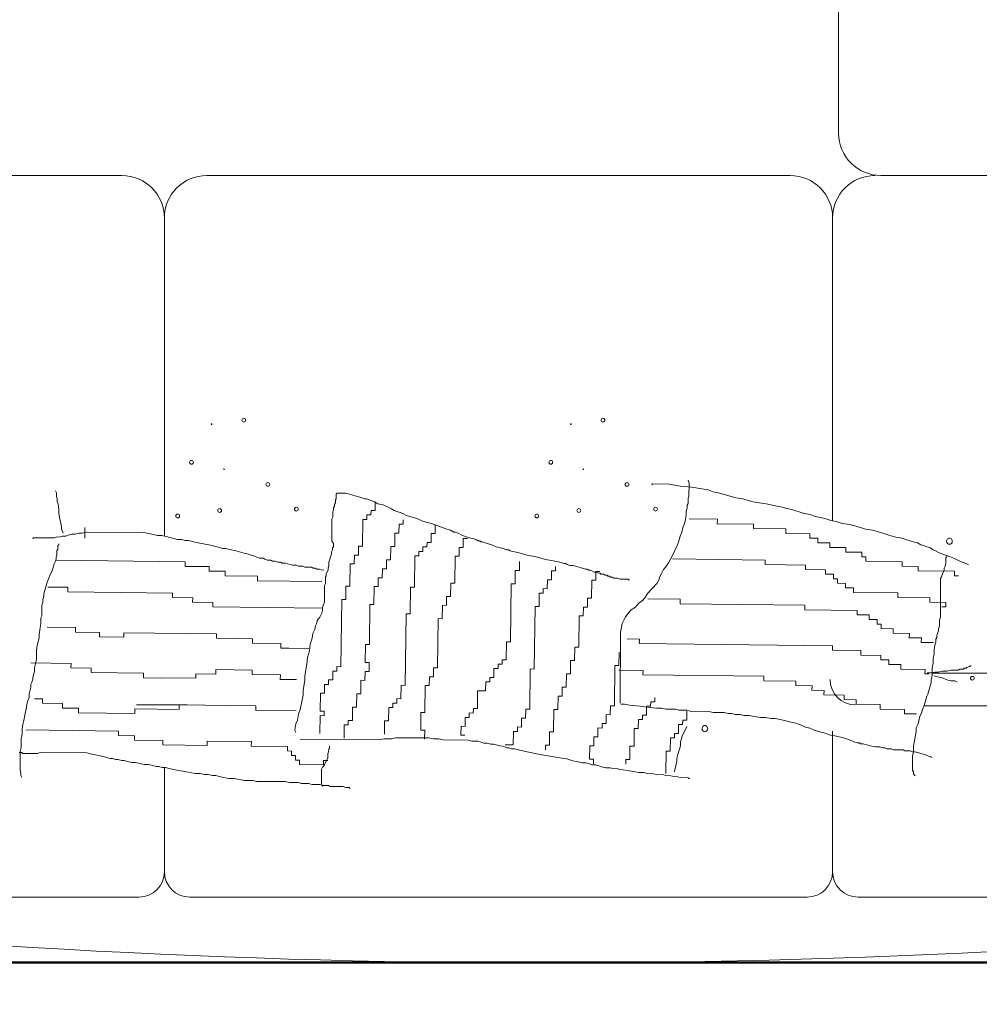
# Model space of a CAD drawing. Units: inches. Extents: x -466983 to 1020, y 324 to 318697.
# Tile 20 of 97: x 721 to 775, y 511 to 566. Entities that reach past the tile are written whole.
import ezdxf

# ---------------------------------------------------------------- set-up
doc = ezdxf.new("R2010")
doc.units = ezdxf.units.IN
doc.header["$MEASUREMENT"] = 0
for name, color, linetype, lineweight in [('A-ANNO-DIMS', 2, 'Continuous', 18), ('A-FURN', 8, 'Continuous', 18), ('A-WALL', 7, 'Continuous', 50)]:
    doc.layers.add(name, color=color, linetype=linetype, lineweight=lineweight)
doc.styles.get("Standard").update_dxf_attribs({"font": 'arial.ttf'})
doc.dimstyles.get("Standard").update_dxf_attribs({"dimtxt": 6, "dimasz": 4, "dimexe": 3, "dimexo": 3, "dimgap": 0.09, "dimtad": 0, "dimtih": 1, "dimtoh": 1, "dimdec": 1, "dimzin": 0, "dimdsep": 46, "dimlunit": 3, "dimtxsty": 'Standard', "dimcen": 0.09, "dimadec": 0, "dimazin": 0, "dimtfac": 1, "dimtdec": 1, "dimtofl": 0, "dimtmove": 0, "dimatfit": 3, "dimfxl": 1, "dimtolj": 1, "dimtzin": 0, "dimarcsym": 0})

# ---------------------------------------------------------------- blocks, each defined once
blk = doc.blocks.new('L Shaped Sofa')
at = {"ltscale": 2}
for p, q in [((2432.683, 769.955), (2432.683, 801.818)), ((2377.232, 767.567), (2392.324, 767.567)), ((2429.959, 767.567), (2397.1, 767.567)), ((2469.187, 767.567), (2435.071, 767.567)), ((2394.712, 747.255), (2394.712, 765.179)), ((2432.347, 748.121), (2432.347, 765.179)), ((2422.162, 750.193), (2423.138, 750.189)), ((2422.21, 750.139), (2422.162, 750.193)), ((2423.138, 750.189), (2423.772, 750.077)), ((2423.772, 750.077), (2424.406, 750.02)), ((2424.26, 750.238), (2424.213, 750.4)), ((2424.256, 749.479), (2424.26, 750.238)), ((2424.406, 750.02), (2424.747, 749.964)), ((2424.747, 749.964), (2425.332, 749.853)), ((2388.636, 749.7), (2388.588, 749.809)), ((2388.634, 749.483), (2388.636, 749.7)), ((2388.683, 749.374), (2388.634, 749.483)), ((2388.682, 749.212), (2388.683, 749.374)), ((2404.346, 749.301), (2404.395, 749.355)), ((2404.395, 749.355), (2404.397, 749.626)), ((2404.397, 749.626), (2404.446, 749.68)), ((2404.446, 749.68), (2404.934, 749.678)), ((2404.934, 749.678), (2405.713, 749.457)), ((2405.713, 749.457), (2406.005, 749.347)), ((2406.005, 749.347), (2406.103, 749.347)), ((2406.103, 749.347), (2406.541, 749.182)), ((2424.205, 749.099), (2424.206, 749.37)), ((2424.206, 749.37), (2424.256, 749.479)), ((2425.332, 749.853), (2425.624, 749.743)), ((2425.624, 749.743), (2425.916, 749.688)), ((2425.916, 749.688), (2426.89, 749.412)), ((2426.89, 749.412), (2427.28, 749.356)), ((2427.28, 749.356), (2427.865, 749.191)), ((2388.729, 749.049), (2388.682, 749.212)), ((2388.776, 748.778), (2388.729, 749.049)), ((2404.245, 748.759), (2404.246, 748.868)), ((2404.246, 748.868), (2404.295, 748.922)), ((2404.295, 749.03), (2404.345, 749.138)), ((2404.295, 748.922), (2404.295, 749.03)), ((2404.345, 749.138), (2404.346, 749.301)), ((2406.541, 749.182), (2406.735, 749.073)), ((2406.579, 748.695), (2406.585, 749.199)), ((2406.735, 749.073), (2407.028, 749.017)), ((2407.028, 749.017), (2407.514, 748.798)), ((2407.514, 748.798), (2407.66, 748.689)), ((2424.104, 748.666), (2424.154, 748.828)), ((2424.154, 748.828), (2424.155, 748.991)), ((2424.155, 748.991), (2424.205, 749.099)), ((2427.865, 749.191), (2428.206, 749.135)), ((2428.206, 749.135), (2428.596, 749.079)), ((2428.596, 749.079), (2429.132, 748.968)), ((2429.132, 748.968), (2429.425, 748.912)), ((2429.425, 748.912), (2429.766, 748.802)), ((2429.766, 748.802), (2430.058, 748.747)), ((2388.775, 748.507), (2388.776, 748.778)), ((2388.822, 748.235), (2388.775, 748.507)), ((2388.917, 747.801), (2388.822, 748.235)), ((2404.144, 748.218), (2404.193, 748.326)), ((2404.193, 748.326), (2404.195, 748.597)), ((2404.195, 748.597), (2404.245, 748.759)), ((2406.119, 748.197), (2406.122, 748.449)), ((2406.122, 748.449), (2406.349, 748.446)), ((2406.349, 748.446), (2406.352, 748.698)), ((2406.352, 748.698), (2406.579, 748.695)), ((2407.66, 748.689), (2407.806, 748.634)), ((2407.806, 748.634), (2408.001, 748.579)), ((2408.001, 748.579), (2408.147, 748.524)), ((2408.147, 748.524), (2408.342, 748.415)), ((2408.342, 748.415), (2408.926, 748.249)), ((2408.926, 748.249), (2409.072, 748.194)), ((2424.053, 748.178), (2424.103, 748.449)), ((2424.103, 748.449), (2424.104, 748.666)), ((2430.058, 748.747), (2430.74, 748.526)), ((2430.74, 748.526), (2431.081, 748.471)), ((2431.081, 748.471), (2431.373, 748.361)), ((2431.373, 748.361), (2431.666, 748.305)), ((2431.666, 748.305), (2431.909, 748.25)), ((2431.909, 748.25), (2432.25, 748.14)), ((2388.916, 747.638), (2388.917, 747.801)), ((2390.234, 747.741), (2390.23, 747.144)), ((2404.136, 746.971), (2404.144, 748.218)), ((2405.873, 746.688), (2405.892, 748.199)), ((2405.892, 748.199), (2406.119, 748.197)), ((2407.924, 747.419), (2407.93, 747.923)), ((2407.93, 747.923), (2408.157, 747.92)), ((2408.157, 747.92), (2408.16, 748.172)), ((2409.072, 748.194), (2409.17, 748.14)), ((2409.17, 748.14), (2409.316, 748.085)), ((2409.316, 748.085), (2409.51, 748.03)), ((2409.51, 748.03), (2409.754, 747.974)), ((2409.754, 747.974), (2410.63, 747.645)), ((2409.966, 747.394), (2409.972, 747.898)), ((2423.853, 747.474), (2423.904, 747.745)), ((2423.904, 747.745), (2424.003, 747.962)), ((2424.003, 747.962), (2424.053, 748.178)), ((2424.269, 748.227), (2425.857, 748.207)), ((2425.857, 748.207), (2425.853, 747.956)), ((2425.853, 747.956), (2427.895, 747.931)), ((2427.895, 747.931), (2427.892, 747.679)), ((2427.892, 747.679), (2429.707, 747.657)), ((2432.25, 748.14), (2432.543, 748.084)), ((2432.543, 748.084), (2432.884, 747.974)), ((2432.884, 747.974), (2433.322, 747.918)), ((2433.322, 747.918), (2433.858, 747.753)), ((2433.858, 747.753), (2434.199, 747.643)), ((2387.302, 747.104), (2387.351, 747.158)), ((2387.351, 747.158), (2388.523, 747.152)), ((2388.523, 747.152), (2388.669, 747.206)), ((2388.669, 747.206), (2388.816, 747.205)), ((2388.816, 747.205), (2388.962, 747.259)), ((2389.012, 747.421), (2388.916, 747.638)), ((2388.962, 747.259), (2389.158, 747.258)), ((2389.158, 747.258), (2389.304, 747.311)), ((2389.304, 747.311), (2389.5, 747.365)), ((2389.5, 747.365), (2389.695, 747.364)), ((2389.695, 747.364), (2389.89, 747.417)), ((2389.89, 747.417), (2390.086, 747.416)), ((2390.086, 747.416), (2390.33, 747.469)), ((2390.33, 747.469), (2393.55, 747.454)), ((2393.55, 747.454), (2393.843, 747.398)), ((2393.843, 747.398), (2394.33, 747.288)), ((2394.33, 747.288), (2394.574, 747.287)), ((2394.574, 747.287), (2394.818, 747.231)), ((2394.818, 747.231), (2395.013, 747.176)), ((2395.013, 747.176), (2395.256, 747.121)), ((2407.688, 746.666), (2407.697, 747.422)), ((2407.697, 747.422), (2407.924, 747.419)), ((2409.733, 746.893), (2409.739, 747.397)), ((2409.739, 747.397), (2409.966, 747.394)), ((2410.63, 747.645), (2410.825, 747.59)), ((2410.825, 747.59), (2411.02, 747.48)), ((2411.02, 747.48), (2411.117, 747.48)), ((2411.117, 747.48), (2411.263, 747.425)), ((2411.263, 747.425), (2411.458, 747.316)), ((2411.458, 747.316), (2411.701, 747.206)), ((2411.544, 746.619), (2411.55, 747.123)), ((2411.55, 747.123), (2411.777, 747.12)), ((2411.701, 747.206), (2411.896, 747.151)), ((2411.896, 747.151), (2412.14, 747.096)), ((2423.704, 747.041), (2423.754, 747.258)), ((2423.754, 747.258), (2423.853, 747.474)), ((2429.707, 747.657), (2429.704, 747.405)), ((2429.704, 747.405), (2431.065, 747.388)), ((2431.065, 747.388), (2431.061, 747.136)), ((2431.061, 747.136), (2431.515, 747.131)), ((2431.515, 747.131), (2431.512, 746.879)), ((2434.199, 747.643), (2434.589, 747.587)), ((2434.589, 747.587), (2435.174, 747.421)), ((2435.174, 747.421), (2435.515, 747.311)), ((2435.515, 747.311), (2435.904, 747.201)), ((2435.904, 747.201), (2436.246, 747.145)), ((2436.246, 747.145), (2436.586, 747.035)), ((2388.714, 746.501), (2388.715, 746.718)), ((2388.715, 746.718), (2388.764, 746.772)), ((2388.764, 746.772), (2388.765, 746.826)), ((2395.256, 747.121), (2395.451, 747.066)), ((2395.451, 747.066), (2395.695, 747.064)), ((2395.695, 747.064), (2395.89, 747.009)), ((2395.89, 747.009), (2396.085, 747.008)), ((2396.085, 747.008), (2396.28, 746.953)), ((2396.28, 746.953), (2396.524, 746.898)), ((2396.524, 746.898), (2397.401, 746.731)), ((2397.401, 746.731), (2397.596, 746.676)), ((2397.596, 746.676), (2397.839, 746.621)), ((2397.839, 746.621), (2397.985, 746.566)), ((2404.233, 746.862), (2404.136, 746.971)), ((2404.182, 746.482), (2404.183, 746.591)), ((2404.183, 746.591), (2404.232, 746.645)), ((2404.232, 746.645), (2404.233, 746.862)), ((2405.64, 746.187), (2405.647, 746.691)), ((2405.647, 746.691), (2405.873, 746.688)), ((2407.452, 745.913), (2407.461, 746.669)), ((2407.461, 746.669), (2407.688, 746.666)), ((2409.273, 746.394), (2409.276, 746.646)), ((2409.276, 746.646), (2409.503, 746.644)), ((2409.503, 746.644), (2409.506, 746.896)), ((2409.506, 746.896), (2409.733, 746.893)), ((2411.311, 746.118), (2411.317, 746.621)), ((2411.317, 746.621), (2411.544, 746.619)), ((2412.14, 747.096), (2412.286, 747.041)), ((2412.286, 747.041), (2412.383, 746.986)), ((2412.383, 746.986), (2412.481, 746.986)), ((2412.481, 746.986), (2412.529, 746.931)), ((2412.529, 746.931), (2412.627, 746.931)), ((2412.627, 746.931), (2412.773, 746.876)), ((2412.773, 746.876), (2413.162, 746.766)), ((2413.162, 746.766), (2413.406, 746.656)), ((2413.406, 746.656), (2413.649, 746.601)), ((2413.649, 746.601), (2413.844, 746.545)), ((2423.308, 746.122), (2423.605, 746.771)), ((2423.605, 746.771), (2423.704, 747.041)), ((2431.512, 746.879), (2432.193, 746.87)), ((2432.193, 746.87), (2432.19, 746.618)), ((2432.19, 746.618), (2433.097, 746.607)), ((2433.097, 746.607), (2433.094, 746.355)), ((2436.586, 747.035), (2436.879, 746.925)), ((2436.879, 746.925), (2437.122, 746.87)), ((2437.122, 746.87), (2437.317, 746.761)), ((2437.317, 746.761), (2437.512, 746.705)), ((2437.512, 746.705), (2437.658, 746.651)), ((2437.658, 746.651), (2437.852, 746.595)), ((2437.852, 746.595), (2437.998, 746.486)), ((2388.613, 745.959), (2388.614, 746.068)), ((2388.614, 746.068), (2388.663, 746.176)), ((2388.663, 746.176), (2388.665, 746.447)), ((2388.665, 746.447), (2388.714, 746.501)), ((2397.985, 746.566), (2398.181, 746.565)), ((2398.181, 746.565), (2398.57, 746.455)), ((2398.57, 746.455), (2398.814, 746.399)), ((2398.814, 746.399), (2399.204, 746.289)), ((2399.204, 746.289), (2399.447, 746.234)), ((2399.447, 746.234), (2399.593, 746.179)), ((2399.593, 746.179), (2399.788, 746.123)), ((2399.788, 746.123), (2400.08, 746.014)), ((2400.08, 746.014), (2400.276, 746.013)), ((2400.276, 746.013), (2400.373, 745.958)), ((2403.983, 745.779), (2404.132, 746.266)), ((2404.132, 746.266), (2404.133, 746.374)), ((2404.133, 746.374), (2404.182, 746.482)), ((2405.407, 745.686), (2405.414, 746.19)), ((2405.414, 746.19), (2405.64, 746.187)), ((2408.795, 744.385), (2408.816, 746.148)), ((2408.816, 746.148), (2409.043, 746.145)), ((2409.043, 746.145), (2409.046, 746.397)), ((2409.046, 746.397), (2409.273, 746.394)), ((2411.066, 744.609), (2411.084, 746.12)), ((2411.084, 746.12), (2411.311, 746.118)), ((2413.844, 746.545), (2413.99, 746.491)), ((2413.99, 746.491), (2414.088, 746.49)), ((2414.088, 746.49), (2414.185, 746.435)), ((2414.185, 746.435), (2414.331, 746.381)), ((2414.331, 746.381), (2414.624, 746.325)), ((2414.624, 746.325), (2415.208, 746.16)), ((2415.208, 746.16), (2415.598, 746.104)), ((2415.598, 746.104), (2416.183, 745.938)), ((2423.21, 745.959), (2423.308, 746.122)), ((2433.094, 746.355), (2434.001, 746.344)), ((2434.001, 746.344), (2433.998, 746.092)), ((2433.998, 746.092), (2434.225, 746.09)), ((2434.225, 746.09), (2434.222, 745.838)), ((2437.998, 746.486), (2438.144, 746.431)), ((2438.144, 746.431), (2438.339, 746.322)), ((2438.339, 746.322), (2438.582, 746.213)), ((2438.582, 746.213), (2438.923, 746.102)), ((2438.725, 745.724), (2438.727, 746.049)), ((2438.727, 746.049), (2438.777, 746.103)), ((2438.923, 746.102), (2439.215, 745.993)), ((2388.414, 745.364), (2388.514, 745.688)), ((2388.514, 745.688), (2388.563, 745.797)), ((2388.563, 745.797), (2388.613, 745.959)), ((2388.622, 745.891), (2395.88, 745.802)), ((2395.88, 745.802), (2395.877, 745.55)), ((2395.877, 745.55), (2397.238, 745.534)), ((2397.238, 745.534), (2397.235, 745.282)), ((2400.373, 745.958), (2400.519, 745.903)), ((2400.519, 745.903), (2400.714, 745.902)), ((2400.714, 745.902), (2400.811, 745.848)), ((2400.811, 745.848), (2400.958, 745.847)), ((2400.958, 745.847), (2401.104, 745.792)), ((2401.104, 745.792), (2401.25, 745.791)), ((2401.25, 745.791), (2401.347, 745.737)), ((2401.347, 745.737), (2401.543, 745.736)), ((2401.543, 745.736), (2401.932, 745.625)), ((2401.932, 745.625), (2402.127, 745.625)), ((2402.127, 745.625), (2402.273, 745.57)), ((2402.273, 745.57), (2402.517, 745.569)), ((2402.517, 745.569), (2402.615, 745.514)), ((2402.615, 745.514), (2403.005, 745.512)), ((2403.005, 745.512), (2403.102, 745.457)), ((2403.102, 745.457), (2403.2, 745.457)), ((2403.2, 745.457), (2403.297, 745.402)), ((2403.932, 745.453), (2403.982, 745.616)), ((2403.982, 745.616), (2403.983, 745.779)), ((2405.165, 744.429), (2405.181, 745.689)), ((2405.181, 745.689), (2405.407, 745.686)), ((2407.219, 745.412), (2407.225, 745.916)), ((2407.225, 745.916), (2407.452, 745.913)), ((2414.705, 745.32), (2414.711, 745.824)), ((2416.183, 745.938), (2416.524, 745.882)), ((2416.524, 745.882), (2416.816, 745.827)), ((2416.746, 745.295), (2416.749, 745.547)), ((2416.816, 745.827), (2417.06, 745.771)), ((2417.06, 745.771), (2417.206, 745.716)), ((2417.206, 745.716), (2417.304, 745.716)), ((2417.304, 745.716), (2417.401, 745.661)), ((2417.401, 745.661), (2417.547, 745.606)), ((2417.547, 745.606), (2417.742, 745.605)), ((2417.742, 745.605), (2418.132, 745.495)), ((2418.132, 745.495), (2418.424, 745.385)), ((2422.816, 745.365), (2422.963, 745.527)), ((2422.963, 745.527), (2423.111, 745.743)), ((2423.111, 745.743), (2423.21, 745.959)), ((2423.334, 745.971), (2428.551, 745.907)), ((2428.551, 745.907), (2428.548, 745.655)), ((2428.548, 745.655), (2430.816, 745.627)), ((2430.816, 745.627), (2430.813, 745.375)), ((2434.222, 745.838), (2436.263, 745.813)), ((2436.263, 745.813), (2436.26, 745.561)), ((2436.26, 745.561), (2437.168, 745.55)), ((2437.168, 745.55), (2437.165, 745.298)), ((2438.626, 745.453), (2438.676, 745.561)), ((2438.676, 745.561), (2438.725, 745.724)), ((2439.215, 745.993), (2439.556, 745.828)), ((2439.556, 745.828), (2439.994, 745.664)), ((2388.216, 744.877), (2388.266, 745.039)), ((2388.266, 745.039), (2388.414, 745.364)), ((2397.235, 745.282), (2398.143, 745.271)), ((2398.143, 745.271), (2398.139, 745.019)), ((2398.139, 745.019), (2399.954, 744.997)), ((2399.954, 744.997), (2399.951, 744.745)), ((2403.297, 745.402), (2403.444, 745.402)), ((2403.444, 745.402), (2403.541, 745.347)), ((2403.541, 745.347), (2403.687, 745.346)), ((2403.78, 744.587), (2403.782, 744.966)), ((2403.782, 744.966), (2403.832, 745.02)), ((2403.832, 745.129), (2403.931, 745.345)), ((2403.832, 745.02), (2403.832, 745.129)), ((2403.931, 745.345), (2403.932, 745.453)), ((2406.753, 744.41), (2406.759, 744.914)), ((2406.759, 744.914), (2406.986, 744.911)), ((2406.986, 744.911), (2406.992, 745.415)), ((2406.992, 745.415), (2407.219, 745.412)), ((2414.469, 744.567), (2414.478, 745.323)), ((2414.478, 745.323), (2414.705, 745.32)), ((2416.513, 744.794), (2416.519, 745.298)), ((2416.519, 745.298), (2416.746, 745.295)), ((2418.424, 745.385), (2418.522, 745.385)), ((2418.522, 745.385), (2418.619, 745.33)), ((2418.619, 745.33), (2418.716, 745.33)), ((2418.716, 745.33), (2418.911, 745.22)), ((2418.911, 745.22), (2419.057, 745.22)), ((2419.008, 744.764), (2419.015, 745.268)), ((2419.015, 745.268), (2419.241, 745.265)), ((2419.057, 745.22), (2419.155, 745.165)), ((2419.155, 745.165), (2419.252, 745.165)), ((2419.252, 745.165), (2419.301, 745.11)), ((2419.301, 745.11), (2419.447, 745.11)), ((2419.447, 745.11), (2419.544, 745.055)), ((2419.544, 745.055), (2419.642, 745.054)), ((2419.642, 745.054), (2419.69, 745)), ((2419.69, 745), (2419.788, 744.999)), ((2419.788, 744.999), (2419.836, 744.945)), ((2419.836, 744.945), (2419.934, 744.945)), ((2419.934, 744.945), (2420.031, 744.89)), ((2422.568, 744.77), (2422.618, 744.986)), ((2422.618, 744.986), (2422.717, 745.148)), ((2422.717, 745.148), (2422.816, 745.365)), ((2430.813, 745.375), (2431.947, 745.362)), ((2431.947, 745.362), (2431.944, 745.11)), ((2431.944, 745.11), (2432.398, 745.104)), ((2432.398, 745.104), (2432.395, 744.852)), ((2437.165, 745.298), (2439.206, 745.273)), ((2438.427, 744.858), (2438.477, 744.966)), ((2438.477, 744.966), (2438.527, 745.128)), ((2438.527, 745.128), (2438.626, 745.345)), ((2438.626, 745.345), (2438.626, 745.453)), ((2439.206, 745.273), (2439.203, 745.021)), ((2439.43, 745.018), (2439.203, 745.021)), ((2439.203, 745.021), (2439.43, 745.018)), ((2387.918, 744.011), (2388.117, 744.66)), ((2388.117, 744.66), (2388.216, 744.877)), ((2388.149, 744.385), (2389.284, 744.371)), ((2389.284, 744.371), (2389.281, 744.119)), ((2399.951, 744.745), (2403.58, 744.7)), ((2403.725, 743.557), (2403.731, 744.478)), ((2403.731, 744.478), (2403.78, 744.587)), ((2404.929, 743.676), (2404.938, 744.432)), ((2404.938, 744.432), (2405.165, 744.429)), ((2406.514, 743.405), (2406.526, 744.412)), ((2406.526, 744.412), (2406.753, 744.41)), ((2408.549, 742.876), (2408.568, 744.388)), ((2408.568, 744.388), (2408.795, 744.385)), ((2410.83, 743.856), (2410.839, 744.612)), ((2410.839, 744.612), (2411.066, 744.609)), ((2414.202, 741.295), (2414.242, 744.57)), ((2414.242, 744.57), (2414.469, 744.567)), ((2416.28, 744.293), (2416.286, 744.797)), ((2416.286, 744.797), (2416.513, 744.794)), ((2418.769, 743.759), (2418.782, 744.767)), ((2418.782, 744.767), (2419.008, 744.764)), ((2420.031, 744.89), (2420.226, 744.889)), ((2420.226, 744.889), (2420.372, 744.834)), ((2420.372, 744.834), (2420.812, 744.832)), ((2420.812, 744.832), (2420.909, 744.777)), ((2421.929, 744.014), (2422.469, 744.607)), ((2422.469, 744.607), (2422.568, 744.77)), ((2432.395, 744.852), (2432.622, 744.849)), ((2432.622, 744.849), (2432.619, 744.598)), ((2432.619, 744.598), (2433.072, 744.592)), ((2433.072, 744.592), (2433.069, 744.34)), ((2438.414, 742.689), (2438.427, 744.858)), ((2387.867, 743.685), (2387.917, 743.848)), ((2387.917, 743.848), (2387.918, 744.011)), ((2389.281, 744.119), (2395.178, 744.047)), ((2395.178, 744.047), (2395.175, 743.795)), ((2395.175, 743.795), (2396.309, 743.781)), ((2410.597, 743.355), (2410.603, 743.859)), ((2410.603, 743.859), (2410.83, 743.856)), ((2415.814, 743.291), (2415.823, 744.047)), ((2415.823, 744.047), (2416.05, 744.044)), ((2416.05, 744.044), (2416.053, 744.296)), ((2416.053, 744.296), (2416.28, 744.293)), ((2421.634, 743.635), (2421.781, 743.797)), ((2421.781, 743.797), (2421.929, 744.014)), ((2433.069, 744.34), (2433.523, 744.335)), ((2433.523, 744.335), (2433.52, 744.083)), ((2433.52, 744.083), (2436.015, 744.052)), ((2436.015, 744.052), (2436.012, 743.8)), ((2436.012, 743.8), (2437.827, 743.778)), ((2387.813, 742.764), (2387.816, 743.36)), ((2387.816, 743.36), (2387.866, 743.523)), ((2387.866, 743.523), (2387.867, 743.685)), ((2396.309, 743.781), (2396.306, 743.53)), ((2396.306, 743.53), (2397.44, 743.516)), ((2397.44, 743.516), (2397.437, 743.264)), ((2397.437, 743.264), (2403.562, 743.189)), ((2403.625, 743.232), (2403.725, 743.557)), ((2404.656, 739.9), (2404.702, 743.679)), ((2404.702, 743.679), (2404.929, 743.676)), ((2406.259, 741.14), (2406.287, 743.408)), ((2406.287, 743.408), (2406.514, 743.405)), ((2410.361, 742.602), (2410.37, 743.358)), ((2410.37, 743.358), (2410.597, 743.355)), ((2415.544, 739.767), (2415.587, 743.294)), ((2415.587, 743.294), (2415.814, 743.291)), ((2418.303, 742.757), (2418.309, 743.261)), ((2418.309, 743.261), (2418.536, 743.258)), ((2418.536, 743.258), (2418.542, 743.762)), ((2418.542, 743.762), (2418.769, 743.759)), ((2420.996, 743.096), (2421.241, 743.258)), ((2421.241, 743.258), (2421.438, 743.474)), ((2421.438, 743.474), (2421.634, 743.635)), ((2421.945, 743.72), (2423.76, 743.698)), ((2423.76, 743.698), (2423.757, 743.446)), ((2423.757, 743.446), (2430.788, 743.36)), ((2430.788, 743.36), (2430.785, 743.108)), ((2437.827, 743.778), (2437.823, 743.526)), ((2437.823, 743.526), (2438.731, 743.515)), ((2438.728, 743.263), (2438.501, 743.266)), ((2438.731, 743.515), (2438.728, 743.263)), ((2387.763, 742.656), (2387.813, 742.764)), ((2403.378, 742.583), (2403.476, 742.69)), ((2403.476, 742.69), (2403.575, 742.907)), ((2403.575, 742.907), (2403.624, 743.069)), ((2403.624, 743.069), (2403.625, 743.232)), ((2408.273, 738.848), (2408.322, 742.879)), ((2408.322, 742.879), (2408.549, 742.876)), ((2418.055, 740.996), (2418.076, 742.76)), ((2418.076, 742.76), (2418.303, 742.757)), ((2420.603, 742.556), (2420.701, 742.718)), ((2420.701, 742.718), (2420.849, 742.934)), ((2420.849, 742.934), (2420.996, 743.096)), ((2430.785, 743.108), (2433.734, 743.072)), ((2433.734, 743.072), (2433.731, 742.82)), ((2433.731, 742.82), (2434.412, 742.812)), ((2434.412, 742.812), (2434.409, 742.56)), ((2438.364, 742.527), (2438.414, 742.689)), ((2387.711, 742.114), (2387.761, 742.331)), ((2387.761, 742.331), (2387.763, 742.656)), ((2403.179, 741.987), (2403.229, 742.204)), ((2403.229, 742.204), (2403.278, 742.312)), ((2403.278, 742.312), (2403.328, 742.474)), ((2403.328, 742.474), (2403.378, 742.583)), ((2410.1, 739.834), (2410.134, 742.605)), ((2410.134, 742.605), (2410.361, 742.602)), ((2420.453, 742.123), (2420.504, 742.339)), ((2420.504, 742.339), (2420.603, 742.556)), ((2434.409, 742.56), (2434.862, 742.555)), ((2434.862, 742.555), (2434.859, 742.303)), ((2434.859, 742.303), (2435.086, 742.3)), ((2435.086, 742.3), (2435.083, 742.048)), ((2438.312, 742.039), (2438.362, 742.201)), ((2438.362, 742.201), (2438.364, 742.527)), ((2387.659, 741.518), (2387.66, 741.735)), ((2387.66, 741.735), (2387.71, 741.951)), ((2387.71, 741.951), (2387.711, 742.114)), ((2388.122, 742.118), (2389.71, 742.098)), ((2389.71, 742.098), (2389.706, 741.847)), ((2389.706, 741.847), (2391.067, 741.83)), ((2391.067, 741.83), (2391.064, 741.578)), ((2391.064, 741.578), (2392.425, 741.561)), ((2392.425, 741.561), (2392.429, 741.813)), ((2392.429, 741.813), (2397.646, 741.75)), ((2397.646, 741.75), (2397.643, 741.498)), ((2403.029, 741.5), (2403.08, 741.771)), ((2403.08, 741.771), (2403.179, 741.987)), ((2420.378, 737.84), (2420.403, 741.852)), ((2420.403, 741.852), (2420.453, 742.123)), ((2435.083, 742.048), (2435.764, 742.04)), ((2435.764, 742.04), (2435.76, 741.788)), ((2435.76, 741.788), (2436.668, 741.777)), ((2436.668, 741.777), (2436.665, 741.525)), ((2438.212, 741.552), (2438.213, 741.66)), ((2438.213, 741.66), (2438.262, 741.768)), ((2438.262, 741.768), (2438.312, 741.931)), ((2438.312, 741.931), (2438.312, 742.039)), ((2387.508, 740.814), (2387.558, 741.084)), ((2387.558, 741.084), (2387.659, 741.518)), ((2397.643, 741.498), (2399.684, 741.473)), ((2399.684, 741.473), (2399.681, 741.221)), ((2399.681, 741.221), (2401.269, 741.201)), ((2401.269, 741.201), (2401.266, 740.949)), ((2402.879, 740.796), (2402.93, 741.175)), ((2402.93, 741.175), (2403.029, 741.5)), ((2406.02, 740.135), (2406.033, 741.143)), ((2406.033, 741.143), (2406.259, 741.14)), ((2413.963, 740.29), (2413.975, 741.298)), ((2413.975, 741.298), (2414.202, 741.295)), ((2420.783, 741.467), (2421.464, 741.459)), ((2421.464, 741.459), (2421.46, 741.207)), ((2421.46, 741.207), (2432.349, 741.074)), ((2432.349, 741.074), (2432.346, 740.822)), ((2436.665, 741.525), (2437.345, 741.516)), ((2437.345, 741.516), (2437.342, 741.265)), ((2437.342, 741.265), (2438.023, 741.256)), ((2438.061, 740.847), (2438.112, 741.118)), ((2438.112, 741.118), (2438.161, 741.281)), ((2438.161, 741.281), (2438.162, 741.443)), ((2438.162, 741.443), (2438.212, 741.552)), ((2387.505, 740.326), (2387.508, 740.814)), ((2401.266, 740.949), (2401.72, 740.944)), ((2401.493, 740.947), (2402.854, 740.93)), ((2401.72, 740.944), (2401.493, 740.947)), ((2402.779, 740.417), (2402.879, 740.796)), ((2417.819, 740.243), (2417.828, 740.999)), ((2417.828, 740.999), (2418.055, 740.996)), ((2420.311, 739.961), (2420.32, 740.717)), ((2432.346, 740.822), (2433.933, 740.802)), ((2433.933, 740.802), (2433.93, 740.55)), ((2433.93, 740.55), (2435.065, 740.536)), ((2435.065, 740.536), (2435.061, 740.285)), ((2438.009, 740.36), (2438.06, 740.631)), ((2438.06, 740.631), (2438.061, 740.847)), ((2387.19, 740.114), (2389.458, 740.086)), ((2387.404, 739.838), (2387.454, 740.055)), ((2387.454, 740.055), (2387.505, 740.326)), ((2389.458, 740.086), (2389.455, 739.834)), ((2402.626, 739.387), (2402.728, 740.037)), ((2402.728, 740.037), (2402.779, 740.417)), ((2406.247, 740.133), (2406.02, 740.135)), ((2406.241, 739.629), (2406.247, 740.133)), ((2413.503, 739.792), (2413.506, 740.044)), ((2413.506, 740.044), (2413.733, 740.041)), ((2413.733, 740.041), (2413.736, 740.293)), ((2413.736, 740.293), (2413.963, 740.29)), ((2417.583, 739.49), (2417.592, 740.246)), ((2417.592, 740.246), (2417.819, 740.243)), ((2420.056, 737.696), (2420.084, 739.964)), ((2420.084, 739.964), (2420.311, 739.961)), ((2435.061, 740.285), (2435.515, 740.279)), ((2435.515, 740.279), (2435.512, 740.027)), ((2435.512, 740.027), (2436.193, 740.019)), ((2436.193, 740.019), (2436.189, 739.767)), ((2437.957, 739.818), (2438.008, 740.089)), ((2438.008, 740.089), (2438.009, 740.36)), ((2439.909, 739.863), (2440.056, 739.916)), ((2440.056, 739.916), (2440.154, 739.97)), ((2387.303, 739.296), (2387.403, 739.621)), ((2387.403, 739.621), (2387.404, 739.838)), ((2389.455, 739.834), (2390.589, 739.82)), ((2390.589, 739.82), (2390.586, 739.568)), ((2390.586, 739.568), (2393.535, 739.532)), ((2393.535, 739.532), (2393.532, 739.28)), ((2396.481, 739.244), (2396.484, 739.496)), ((2396.484, 739.496), (2397.618, 739.482)), ((2397.618, 739.482), (2397.621, 739.734)), ((2397.621, 739.734), (2399.663, 739.709)), ((2399.663, 739.709), (2399.66, 739.457)), ((2399.66, 739.457), (2401.247, 739.438)), ((2401.247, 739.438), (2401.244, 739.186)), ((2402.624, 739.116), (2402.626, 739.387)), ((2404.193, 739.15), (2404.199, 739.654)), ((2404.199, 739.654), (2404.426, 739.651)), ((2404.426, 739.651), (2404.429, 739.903)), ((2404.429, 739.903), (2404.656, 739.9)), ((2406.008, 739.128), (2406.014, 739.632)), ((2406.014, 739.632), (2406.241, 739.629)), ((2409.867, 739.333), (2409.873, 739.836)), ((2409.873, 739.836), (2410.1, 739.834)), ((2413.27, 739.291), (2413.276, 739.795)), ((2413.276, 739.795), (2413.503, 739.792)), ((2415.29, 737.503), (2415.317, 739.77)), ((2415.317, 739.77), (2415.544, 739.767)), ((2417.347, 738.737), (2417.356, 739.493)), ((2417.356, 739.493), (2417.583, 739.49)), ((2420.308, 739.709), (2421.669, 739.692)), ((2421.669, 739.692), (2421.666, 739.44)), ((2421.666, 739.44), (2428.471, 739.357)), ((2428.471, 739.357), (2428.468, 739.105)), ((2436.189, 739.767), (2437.55, 739.75)), ((2437.55, 739.75), (2437.547, 739.498)), ((2437.547, 739.498), (2437.774, 739.496)), ((2437.663, 739.548), (2437.907, 739.547)), ((2437.905, 739.167), (2437.955, 739.384)), ((2437.907, 739.547), (2438.102, 739.6)), ((2437.955, 739.384), (2437.957, 739.818)), ((2458.96, 739.532), (2437.956, 739.532)), ((2438.052, 739.384), (2438.247, 739.328)), ((2438.102, 739.6), (2438.298, 739.599)), ((2438.298, 739.599), (2438.542, 739.652)), ((2438.542, 739.652), (2438.786, 739.651)), ((2438.786, 739.651), (2439.03, 739.704)), ((2439.03, 739.704), (2439.42, 739.702)), ((2439.42, 739.702), (2439.518, 739.756)), ((2439.518, 739.756), (2439.714, 739.755)), ((2439.714, 739.755), (2439.763, 739.809)), ((2439.763, 739.809), (2439.86, 739.809)), ((2439.86, 739.809), (2439.909, 739.863)), ((2387.202, 738.755), (2387.203, 738.917)), ((2387.203, 738.917), (2387.253, 739.026)), ((2387.253, 739.026), (2387.303, 739.188)), ((2387.303, 739.188), (2387.303, 739.296)), ((2393.532, 739.28), (2396.481, 739.244)), ((2394.569, 739.178), (2394.569, 739.178)), ((2401.244, 739.186), (2402.152, 739.175)), ((2402.523, 738.574), (2402.624, 739.116)), ((2403.73, 738.4), (2403.736, 738.904)), ((2403.736, 738.904), (2403.963, 738.901)), ((2403.963, 738.901), (2403.966, 739.153)), ((2403.966, 739.153), (2404.193, 739.15)), ((2405.772, 738.375), (2405.781, 739.131)), ((2405.781, 739.131), (2406.008, 739.128)), ((2408.037, 738.095), (2408.046, 738.851)), ((2408.046, 738.851), (2408.273, 738.848)), ((2409.389, 737.323), (2409.407, 738.834)), ((2409.407, 738.834), (2409.634, 738.832)), ((2409.634, 738.832), (2409.64, 739.335)), ((2409.64, 739.335), (2409.867, 739.333)), ((2412.807, 738.541), (2412.813, 739.045)), ((2412.813, 739.045), (2413.04, 739.042)), ((2413.04, 739.042), (2413.043, 739.294)), ((2413.043, 739.294), (2413.27, 739.291)), ((2428.468, 739.105), (2430.282, 739.083)), ((2430.282, 739.083), (2430.279, 738.831)), ((2430.279, 738.831), (2431.187, 738.82)), ((2431.187, 738.82), (2431.184, 738.568)), ((2437.704, 738.355), (2437.904, 739.005)), ((2437.904, 739.005), (2437.905, 739.167)), ((2438.247, 739.328), (2438.54, 739.273)), ((2438.54, 739.273), (2438.783, 739.163)), ((2438.783, 739.163), (2439.026, 739.108)), ((2439.026, 739.108), (2439.222, 739.107)), ((2439.222, 739.107), (2439.368, 739.052)), ((2387.101, 738.159), (2387.103, 738.376)), ((2387.103, 738.376), (2387.153, 738.592)), ((2387.153, 738.592), (2387.202, 738.755)), ((2402.37, 737.491), (2402.522, 738.303)), ((2402.522, 738.303), (2402.523, 738.574)), ((2403.491, 737.395), (2403.503, 738.403)), ((2403.503, 738.403), (2403.73, 738.4)), ((2405.536, 737.622), (2405.545, 738.378)), ((2405.545, 738.378), (2405.772, 738.375)), ((2412.341, 737.539), (2412.353, 738.546)), ((2412.353, 738.546), (2412.807, 738.541)), ((2417.114, 738.236), (2417.12, 738.74)), ((2417.12, 738.74), (2417.347, 738.737)), ((2431.184, 738.568), (2431.864, 738.56)), ((2431.864, 738.56), (2431.861, 738.308)), ((2431.861, 738.308), (2432.995, 738.294)), ((2432.995, 738.294), (2432.992, 738.042)), ((2437.605, 738.03), (2437.655, 738.247)), ((2437.655, 738.247), (2437.704, 738.355)), ((2386.8, 736.859), (2387.002, 737.942)), ((2387.002, 737.942), (2387.101, 738.159)), ((2387.392, 738.096), (2387.846, 738.09)), ((2387.846, 738.09), (2387.843, 737.838)), ((2387.843, 737.838), (2388.977, 737.824)), ((2388.977, 737.824), (2388.974, 737.572)), ((2396.001, 737.746), (2393.136, 737.746)), ((2395.552, 737.492), (2395.555, 737.744)), ((2395.555, 737.744), (2399.865, 737.691)), ((2407.577, 737.597), (2407.58, 737.849)), ((2407.58, 737.849), (2407.807, 737.846)), ((2407.807, 737.846), (2407.81, 738.098)), ((2407.81, 738.098), (2408.037, 738.095)), ((2416.878, 737.483), (2416.887, 738.239)), ((2416.887, 738.239), (2417.114, 738.236)), ((2419.823, 737.195), (2419.83, 737.699)), ((2419.83, 737.699), (2420.056, 737.696)), ((2420.427, 737.786), (2420.622, 737.785)), ((2420.622, 737.785), (2420.915, 737.729)), ((2420.915, 737.729), (2421.5, 737.672)), ((2422.098, 737.672), (2422.101, 737.923)), ((2422.101, 737.923), (2422.328, 737.921)), ((2422.328, 737.921), (2422.331, 738.173)), ((2432.992, 738.042), (2433.673, 738.034)), ((2433.673, 738.034), (2433.67, 737.782)), ((2433.67, 737.782), (2435.031, 737.765)), ((2435.031, 737.765), (2435.028, 737.514)), ((2437.406, 737.489), (2437.505, 737.705)), ((2460.8, 737.692), (2437.499, 737.692)), ((2437.505, 737.705), (2437.605, 738.03)), ((2388.974, 737.572), (2389.881, 737.561)), ((2389.881, 737.561), (2389.878, 737.309)), ((2389.878, 737.309), (2393.054, 737.271)), ((2393.054, 737.271), (2393.057, 737.522)), ((2393.057, 737.522), (2395.552, 737.492)), ((2399.865, 737.691), (2399.862, 737.439)), ((2399.862, 737.439), (2402.13, 737.412)), ((2402.22, 736.895), (2402.271, 737.22)), ((2402.271, 737.22), (2402.37, 737.491)), ((2403.476, 736.135), (2403.488, 737.143)), ((2403.488, 737.143), (2403.715, 737.14)), ((2403.718, 737.392), (2403.491, 737.395)), ((2403.715, 737.14), (2403.718, 737.392)), ((2405.3, 736.869), (2405.309, 737.625)), ((2405.309, 737.625), (2405.536, 737.622)), ((2407.341, 736.844), (2407.35, 737.6)), ((2407.35, 737.6), (2407.577, 737.597)), ((2409.15, 736.318), (2409.162, 737.326)), ((2409.162, 737.326), (2409.389, 737.323)), ((2411.881, 737.041), (2411.884, 737.292)), ((2411.884, 737.292), (2412.111, 737.29)), ((2412.111, 737.29), (2412.114, 737.542)), ((2412.114, 737.542), (2412.341, 737.539)), ((2415.057, 737.002), (2415.063, 737.506)), ((2415.063, 737.506), (2415.29, 737.503)), ((2416.635, 736.227), (2416.651, 737.486)), ((2416.651, 737.486), (2416.878, 737.483)), ((2419.59, 736.694), (2419.597, 737.198)), ((2419.597, 737.198), (2419.823, 737.195)), ((2421.5, 737.672), (2421.89, 737.616)), ((2421.635, 736.921), (2421.638, 737.173)), ((2421.638, 737.173), (2421.865, 737.17)), ((2421.865, 737.17), (2421.871, 737.674)), ((2421.871, 737.674), (2422.098, 737.672)), ((2421.89, 737.616), (2422.426, 737.559)), ((2422.426, 737.559), (2422.719, 737.558)), ((2422.719, 737.558), (2422.963, 737.503)), ((2422.963, 737.503), (2423.499, 737.5)), ((2423.499, 737.5), (2423.694, 737.445)), ((2423.694, 737.445), (2424.133, 737.443)), ((2424.13, 736.891), (2424.136, 737.395)), ((2424.133, 737.443), (2424.328, 737.388)), ((2424.328, 737.388), (2425.353, 737.383)), ((2425.353, 737.383), (2425.645, 737.327)), ((2425.645, 737.327), (2426.231, 737.325)), ((2426.231, 737.325), (2426.475, 737.269)), ((2426.475, 737.269), (2426.67, 737.268)), ((2426.67, 737.268), (2426.865, 737.213)), ((2426.865, 737.213), (2427.157, 737.212)), ((2427.157, 737.212), (2427.352, 737.157)), ((2427.352, 737.157), (2427.645, 737.155)), ((2427.645, 737.155), (2427.937, 737.1)), ((2435.028, 737.514), (2436.389, 737.497)), ((2436.389, 737.497), (2436.386, 737.245)), ((2436.386, 737.245), (2437.066, 737.237)), ((2437.258, 737.11), (2437.356, 737.272)), ((2437.356, 737.272), (2437.406, 737.489)), ((2386.7, 736.372), (2386.75, 736.642)), ((2386.75, 736.642), (2386.8, 736.859)), ((2402.071, 736.462), (2402.121, 736.679)), ((2402.121, 736.679), (2402.22, 736.895)), ((2404.834, 735.867), (2404.843, 736.623)), ((2404.843, 736.623), (2405.07, 736.62)), ((2405.07, 736.62), (2405.073, 736.872)), ((2405.073, 736.872), (2405.3, 736.869)), ((2407.105, 736.091), (2407.114, 736.847)), ((2407.114, 736.847), (2407.341, 736.844)), ((2411.648, 736.539), (2411.654, 737.043)), ((2411.654, 737.043), (2411.881, 737.041)), ((2414.824, 736.501), (2414.83, 737.004)), ((2414.83, 737.004), (2415.057, 737.002)), ((2419.36, 736.445), (2419.364, 736.697)), ((2419.364, 736.697), (2419.59, 736.694)), ((2421.402, 736.42), (2421.408, 736.924)), ((2421.408, 736.924), (2421.635, 736.921)), ((2423.667, 736.141), (2423.673, 736.644)), ((2423.673, 736.644), (2423.9, 736.642)), ((2423.9, 736.642), (2423.903, 736.894)), ((2423.903, 736.894), (2424.13, 736.891)), ((2427.937, 737.1), (2428.279, 737.044)), ((2428.279, 737.044), (2428.571, 737.043)), ((2428.571, 737.043), (2428.864, 736.987)), ((2428.864, 736.987), (2429.108, 736.986)), ((2429.108, 736.986), (2429.4, 736.93)), ((2429.4, 736.93), (2429.644, 736.875)), ((2429.644, 736.875), (2429.985, 736.765)), ((2429.985, 736.765), (2430.277, 736.709)), ((2430.277, 736.709), (2430.569, 736.599)), ((2430.569, 736.599), (2430.813, 736.49)), ((2437.058, 736.461), (2437.157, 736.677)), ((2437.157, 736.677), (2437.258, 737.11)), ((2386.648, 735.83), (2386.698, 736.101)), ((2386.698, 736.101), (2386.7, 736.372)), ((2386.917, 736.338), (2392.134, 736.274)), ((2392.134, 736.274), (2392.131, 736.022)), ((2402.07, 736.299), (2402.071, 736.462)), ((2402.118, 736.191), (2402.07, 736.299)), ((2409.377, 736.315), (2409.15, 736.318)), ((2409.37, 735.811), (2409.377, 736.315)), ((2411.415, 736.038), (2411.421, 736.542)), ((2411.642, 736.036), (2411.415, 736.038)), ((2411.421, 736.542), (2411.648, 736.539)), ((2414.358, 735.499), (2414.367, 736.254)), ((2414.367, 736.254), (2414.594, 736.252)), ((2414.594, 736.252), (2414.597, 736.503)), ((2414.597, 736.503), (2414.824, 736.501)), ((2416.399, 735.474), (2416.409, 736.229)), ((2416.409, 736.229), (2416.635, 736.227)), ((2419.127, 735.944), (2419.134, 736.448)), ((2419.134, 736.448), (2419.36, 736.445)), ((2421.163, 735.415), (2421.175, 736.423)), ((2421.175, 736.423), (2421.402, 736.42)), ((2423.437, 735.892), (2423.44, 736.143)), ((2423.44, 736.143), (2423.667, 736.141)), ((2423.88, 735.98), (2424.128, 736.521)), ((2430.813, 736.49), (2431.056, 736.434)), ((2431.056, 736.434), (2431.3, 736.325)), ((2431.3, 736.325), (2431.689, 736.215)), ((2431.689, 736.215), (2431.933, 736.159)), ((2431.933, 736.159), (2432.225, 736.049)), ((2432.225, 736.049), (2432.566, 735.994)), ((2432.347, 728.35), (2432.347, 736.259)), ((2436.906, 735.431), (2437.057, 736.244)), ((2437.057, 736.244), (2437.058, 736.461)), ((2386.645, 735.342), (2386.648, 735.83)), ((2392.131, 736.022), (2393.038, 736.011)), ((2393.038, 736.011), (2393.035, 735.759)), ((2393.035, 735.759), (2394.623, 735.74)), ((2394.623, 735.74), (2394.62, 735.488)), ((2394.62, 735.488), (2397.115, 735.457)), ((2397.115, 735.457), (2397.118, 735.709)), ((2397.118, 735.709), (2399.613, 735.679)), ((2399.613, 735.679), (2399.61, 735.427)), ((2402.36, 735.81), (2406.898, 735.789)), ((2406.898, 735.789), (2407.094, 735.842)), ((2407.094, 735.842), (2407.533, 735.84)), ((2407.533, 735.84), (2407.728, 735.893)), ((2407.728, 735.893), (2409.582, 735.885)), ((2409.582, 735.885), (2409.875, 735.829)), ((2409.875, 735.829), (2410.168, 735.828)), ((2410.168, 735.828), (2410.411, 735.772)), ((2410.411, 735.772), (2411.826, 735.766)), ((2411.826, 735.766), (2412.021, 735.711)), ((2412.021, 735.711), (2412.363, 735.709)), ((2412.363, 735.709), (2412.558, 735.654)), ((2412.558, 735.654), (2412.704, 735.599)), ((2412.704, 735.599), (2412.899, 735.598)), ((2412.899, 735.598), (2413.094, 735.543)), ((2413.094, 735.543), (2413.24, 735.542)), ((2413.24, 735.542), (2413.63, 735.432)), ((2413.904, 735.504), (2414.358, 735.499)), ((2416.169, 735.224), (2416.172, 735.476)), ((2416.172, 735.476), (2416.399, 735.474)), ((2418.895, 735.443), (2418.901, 735.947)), ((2418.901, 735.947), (2419.127, 735.944)), ((2423.201, 735.139), (2423.211, 735.894)), ((2423.211, 735.894), (2423.437, 735.892)), ((2423.78, 735.439), (2423.781, 735.655)), ((2423.781, 735.655), (2423.88, 735.98)), ((2432.566, 735.994), (2432.956, 735.883)), ((2432.956, 735.883), (2433.297, 735.773)), ((2433.297, 735.773), (2433.54, 735.664)), ((2433.54, 735.664), (2433.735, 735.609)), ((2433.735, 735.609), (2433.833, 735.608)), ((2433.833, 735.608), (2433.93, 735.554)), ((2433.93, 735.554), (2434.076, 735.553)), ((2434.076, 735.553), (2434.466, 735.443)), ((2386.546, 735.071), (2386.692, 735.07)), ((2386.588, 734.095), (2386.595, 735.125)), ((2386.595, 735.125), (2386.645, 735.342)), ((2386.692, 735.07), (2386.74, 735.016)), ((2386.74, 735.016), (2387.57, 735.012)), ((2387.57, 735.012), (2387.717, 735.066)), ((2387.717, 735.066), (2390.352, 735.053)), ((2390.352, 735.053), (2390.546, 734.998)), ((2390.546, 734.998), (2391.277, 734.832)), ((2399.61, 735.427), (2401.652, 735.402)), ((2401.652, 735.402), (2401.649, 735.15)), ((2401.649, 735.15), (2401.876, 735.147)), ((2401.876, 735.147), (2401.873, 734.895)), ((2403.915, 734.773), (2403.917, 734.99)), ((2403.917, 734.99), (2403.966, 735.098)), ((2403.966, 735.098), (2403.967, 735.26)), ((2403.967, 735.26), (2404.016, 735.314)), ((2404.016, 735.314), (2404.017, 735.423)), ((2413.63, 735.432), (2413.776, 735.431)), ((2413.776, 735.431), (2413.873, 735.377)), ((2413.873, 735.377), (2414.019, 735.322)), ((2414.019, 735.322), (2414.117, 735.321)), ((2414.117, 735.321), (2414.263, 735.266)), ((2414.263, 735.266), (2414.458, 735.265)), ((2414.458, 735.265), (2414.653, 735.21)), ((2414.653, 735.21), (2415.14, 735.1)), ((2415.14, 735.1), (2415.433, 735.044)), ((2415.433, 735.044), (2415.677, 734.989)), ((2415.677, 734.989), (2415.969, 734.933)), ((2415.969, 734.933), (2416.993, 734.766)), ((2418.658, 734.69), (2418.668, 735.446)), ((2418.668, 735.446), (2418.895, 735.443)), ((2420.927, 734.662), (2420.936, 735.418)), ((2420.936, 735.418), (2421.163, 735.415)), ((2422.959, 733.882), (2422.974, 735.141)), ((2422.974, 735.141), (2423.201, 735.139)), ((2423.58, 734.735), (2423.63, 734.951)), ((2423.63, 734.951), (2423.78, 735.439)), ((2434.466, 735.443), (2434.758, 735.387)), ((2434.758, 735.387), (2435.002, 735.386)), ((2435.002, 735.386), (2435.197, 735.331)), ((2435.197, 735.331), (2435.295, 735.33)), ((2435.295, 735.33), (2435.392, 735.276)), ((2435.392, 735.276), (2435.636, 735.274)), ((2435.636, 735.274), (2435.782, 735.22)), ((2435.782, 735.22), (2436.319, 735.217)), ((2436.319, 735.217), (2436.416, 735.162)), ((2436.416, 735.162), (2436.709, 735.161)), ((2436.709, 735.161), (2436.855, 735.106)), ((2436.853, 734.835), (2436.904, 735.16)), ((2436.855, 735.106), (2437.001, 735.105)), ((2436.904, 735.16), (2436.906, 735.431)), ((2437.001, 735.105), (2437.586, 734.94)), ((2437.586, 734.94), (2437.78, 734.831)), ((2391.277, 734.832), (2391.667, 734.722)), ((2391.667, 734.722), (2391.813, 734.721)), ((2391.813, 734.721), (2391.959, 734.666)), ((2391.959, 734.666), (2392.106, 734.665)), ((2392.106, 734.665), (2392.301, 734.61)), ((2392.301, 734.61), (2392.447, 734.61)), ((2392.447, 734.61), (2392.642, 734.555)), ((2392.642, 734.555), (2392.886, 734.499)), ((2392.886, 734.499), (2393.081, 734.498)), ((2393.081, 734.498), (2393.568, 734.388)), ((2393.568, 734.388), (2393.812, 734.386)), ((2393.812, 734.386), (2394.056, 734.331)), ((2401.873, 734.895), (2402.099, 734.892)), ((2402.099, 734.892), (2402.096, 734.641)), ((2402.096, 734.641), (2402.323, 734.638)), ((2402.323, 734.638), (2402.32, 734.386)), ((2402.32, 734.386), (2403.681, 734.369)), ((2403.681, 734.369), (2403.684, 734.621)), ((2403.684, 734.621), (2403.911, 734.618)), ((2403.717, 734.34), (2403.915, 734.773)), ((2416.993, 734.766), (2417.383, 734.709)), ((2417.383, 734.709), (2417.724, 734.599)), ((2417.724, 734.599), (2418.016, 734.544)), ((2418.016, 734.544), (2418.26, 734.488)), ((2418.26, 734.488), (2418.455, 734.488)), ((2418.455, 734.488), (2418.65, 734.432)), ((2418.65, 734.432), (2418.796, 734.378)), ((2418.885, 734.687), (2418.658, 734.69)), ((2418.796, 734.378), (2418.991, 734.377)), ((2418.882, 734.435), (2418.885, 734.687)), ((2418.991, 734.377), (2419.186, 734.321)), ((2420.697, 734.413), (2420.7, 734.665)), ((2420.7, 734.665), (2420.927, 734.662)), ((2423.479, 734.139), (2423.579, 734.572)), ((2423.579, 734.572), (2423.58, 734.735)), ((2436.849, 734.076), (2436.853, 734.835)), ((2437.78, 734.831), (2437.878, 734.83)), ((2437.878, 734.83), (2437.926, 734.776)), ((2386.636, 733.878), (2386.588, 734.095)), ((2386.635, 733.769), (2386.636, 733.878)), ((2394.056, 734.331), (2394.25, 734.276)), ((2394.25, 734.276), (2394.397, 734.275)), ((2394.397, 734.275), (2394.592, 734.22)), ((2394.592, 734.22), (2394.787, 734.219)), ((2394.712, 728.35), (2394.712, 734.219)), ((2394.787, 734.219), (2394.982, 734.164)), ((2394.982, 734.164), (2395.225, 734.109)), ((2395.225, 734.109), (2395.518, 734.053)), ((2395.518, 734.053), (2395.859, 733.997)), ((2395.859, 733.997), (2396.444, 733.886)), ((2396.444, 733.886), (2396.737, 733.885)), ((2396.737, 733.885), (2396.98, 733.829)), ((2396.98, 733.829), (2397.176, 733.828)), ((2397.176, 733.828), (2397.419, 733.773)), ((2403.565, 733.31), (2403.57, 734.124)), ((2403.57, 734.124), (2403.619, 734.232)), ((2403.619, 734.232), (2403.717, 734.34)), ((2419.186, 734.321), (2419.332, 734.267)), ((2419.332, 734.267), (2419.575, 734.211)), ((2419.575, 734.211), (2419.819, 734.21)), ((2419.819, 734.21), (2419.966, 734.155)), ((2419.966, 734.155), (2420.258, 734.154)), ((2420.258, 734.154), (2420.356, 734.099)), ((2420.356, 734.099), (2420.551, 734.098)), ((2420.551, 734.098), (2420.794, 734.043)), ((2420.794, 734.043), (2421.136, 733.987)), ((2421.136, 733.987), (2421.428, 733.931)), ((2421.428, 733.931), (2421.721, 733.93)), ((2421.721, 733.93), (2421.916, 733.875)), ((2421.916, 733.875), (2422.257, 733.873)), ((2422.257, 733.873), (2422.403, 733.818)), ((2422.403, 733.818), (2422.842, 733.816)), ((2422.842, 733.816), (2422.94, 733.762)), ((2423.429, 733.976), (2423.479, 734.139)), ((2436.897, 733.967), (2436.849, 734.076)), ((2436.896, 733.859), (2436.897, 733.967)), ((2436.993, 733.75), (2436.896, 733.859)), ((2386.683, 733.661), (2386.635, 733.769)), ((2397.419, 733.773), (2397.614, 733.772)), ((2397.614, 733.772), (2397.809, 733.717)), ((2397.809, 733.717), (2398.053, 733.662)), ((2398.053, 733.662), (2398.345, 733.606)), ((2398.345, 733.606), (2398.638, 733.605)), ((2398.638, 733.605), (2399.223, 733.493)), ((2399.223, 733.493), (2399.711, 733.491)), ((2399.711, 733.491), (2399.906, 733.436)), ((2399.906, 733.436), (2401.516, 733.429)), ((2401.516, 733.429), (2401.76, 733.373)), ((2401.76, 733.373), (2402.248, 733.371)), ((2402.248, 733.371), (2402.442, 733.316)), ((2402.442, 733.316), (2402.833, 733.314)), ((2402.833, 733.314), (2403.028, 733.259)), ((2403.028, 733.259), (2403.467, 733.257)), ((2403.467, 733.257), (2403.613, 733.202)), ((2403.613, 733.148), (2403.565, 733.31)), ((2422.94, 733.762), (2423.232, 733.76)), ((2423.232, 733.76), (2423.427, 733.705)), ((2423.427, 733.705), (2423.622, 733.704)), ((2423.622, 733.704), (2423.769, 733.649)), ((2423.769, 733.649), (2424.208, 733.647)), ((2424.208, 733.647), (2424.256, 733.593)), ((2424.256, 733.593), (2424.305, 733.593)), ((2403.613, 733.202), (2403.954, 733.2)), ((2403.954, 733.2), (2404.052, 733.146)), ((2404.052, 733.146), (2404.784, 733.142)), ((2404.784, 733.142), (2404.93, 733.087)), ((2404.93, 733.087), (2405.125, 733.086)), ((2405.125, 733.086), (2405.173, 733.032)), ((2393.28, 726.917), (2377.232, 726.917)), ((2430.914, 726.917), (2396.145, 726.917)), ((2469.187, 726.917), (2433.78, 726.917)), ((2475.263, 723.229), (2377.232, 723.229))]:
    blk.add_line(p, q, dxfattribs=at)
for centre, radius, start, end in [((2435.071, 769.955), 2.388, 180, 270), ((2392.324, 765.179), 2.388, 0, 90), ((2397.1, 765.179), 2.388, 90, 180), ((2429.959, 765.179), 2.388, 0, 90), ((2434.735, 765.179), 2.388, 90, 180), ((2399.184, 753.788), 0.106, 90, 270), ((2399.184, 753.788), 0.106, 270, 90), ((2419.413, 753.788), 0.106, 90, 270), ((2419.413, 753.788), 0.106, 270, 90), ((2397.375, 753.562), 0.0177, 90, 270), ((2397.375, 753.562), 0.0177, 270, 90), ((2417.604, 753.562), 0.0177, 90, 270), ((2417.604, 753.562), 0.0177, 270, 90), ((2396.244, 751.412), 0.106, 90, 270), ((2396.244, 751.412), 0.106, 270, 90), ((2398.074, 751.018), 0.0177, 90, 270), ((2398.074, 751.018), 0.0177, 270, 90), ((2416.474, 751.412), 0.106, 90, 270), ((2416.474, 751.412), 0.106, 270, 90), ((2418.303, 751.018), 0.0177, 90, 270), ((2418.303, 751.018), 0.0177, 270, 90), ((2400.541, 750.168), 0.106, 90, 270), ((2400.541, 750.168), 0.106, 270, 90), ((2420.77, 750.168), 0.106, 90, 270), ((2420.77, 750.168), 0.106, 270, 90), ((2397.827, 748.697), 0.106, 90, 270), ((2397.827, 748.697), 0.106, 270, 90), ((2402.147, 748.771), 0.106, 90, 270), ((2402.147, 748.771), 0.106, 270, 90), ((2418.057, 748.697), 0.106, 90, 270), ((2418.057, 748.697), 0.106, 270, 90), ((2422.376, 748.771), 0.106, 90, 270), ((2422.376, 748.771), 0.106, 270, 90), ((2395.463, 748.389), 0.106, 90, 270), ((2395.463, 748.389), 0.106, 270, 90), ((2415.692, 748.389), 0.106, 90, 270), ((2415.692, 748.389), 0.106, 270, 90), ((2440.217, 739.25), 0.106, 90, 270), ((2440.217, 739.25), 0.106, 270, 90), ((2433.636, 739.178), 1.433, 180, 270), ((2393.28, 728.35), 1.433, 270, 0), ((2396.145, 728.35), 1.433, 180, 270), ((2430.914, 728.35), 1.433, 270, 0), ((2433.78, 728.35), 1.433, 180, 270), ((2416.36, 1205.029), 481.82, 262.88673, 276.63201)]:
    blk.add_arc(centre, radius, start, end, dxfattribs=at)
at = {"ltscale": 2, "extrusion": (0, 0, -1)}
for centre, start_param, end_param in [((2438.928, 746.97), 1.570796, 4.712389), ((2438.928, 746.97), -1.570796, 1.570796), ((2425.152, 736.408), 1.570796, 4.712389), ((2425.152, 736.408), -1.570796, 1.570796)]:
    blk.add_ellipse(centre, major_axis=(-0.002, -0.177), ratio=0.9, start_param=start_param, end_param=end_param, dxfattribs=at)
blk = doc.blocks.new('*D70')
at = {"layer": 'A-ANNO-DIMS', "color": 0, "lineweight": -2, "transparency": 16777216}
for p, q in [((689.806, 508.686), (689.806, 490.005)), ((810.968, 508.686), (810.968, 490.005)), ((693.806, 493.005), (744.53, 493.005)), ((806.968, 493.005), (756.244, 493.005))]:
    blk.add_line(p, q, dxfattribs=at)
at = {"layer": 'A-ANNO-DIMS', "color": 0, "transparency": 16777216}
for points in [[(693.806, 493.671), (693.806, 492.338), (689.806, 493.005)], [(806.968, 493.671), (806.968, 492.338), (810.968, 493.005)]]:
    blk.add_solid(points, dxfattribs=at)
at = {"layer": 'Defpoints', "color": 0, "transparency": 16777216}
for p in [(689.806, 511.686), (810.968, 511.686), (810.968, 493.005)]:
    blk.add_point(p, dxfattribs=at)
at = {"layer": 'A-ANNO-DIMS', "color": 0, "transparency": 16777216, "insert": (750.387, 493.005), "char_height": 6, "attachment_point": 5}
blk.add_mtext('\\A1;121', dxfattribs=at)

msp = doc.modelspace()

# ---------------------------------------------------------------- linework, layer by layer
at = {"layer": 'A-WALL'}
msp.add_line((809.806, 512.938), (660.806, 512.938), dxfattribs=at)

# ---------------------------------------------------------------- block references
at = {"layer": 'A-FURN'}
msp.add_blockref('L Shaped Sofa', (-1665.457, -210.292), dxfattribs=at)

# ---------------------------------------------------------------- dimensions: what is measured, and where the dimension line sits
at = {"layer": 'A-ANNO-DIMS'}
dim = msp.add_linear_dim(base=(810.968, 493.005), p1=(689.806, 511.686), p2=(810.968, 511.686), dimstyle='Standard', override={"dimdec": 0, "dimlfac": 1, "dimrnd": 0, "dimzin": 0, "dimdsep": 46, "dimlunit": 2}, dxfattribs=at)
dim.commit()
dim.dimension.update_dxf_attribs({"geometry": '*D70', "text_midpoint": (750.387, 493.005)})

doc.saveas('drawing.dxf')
